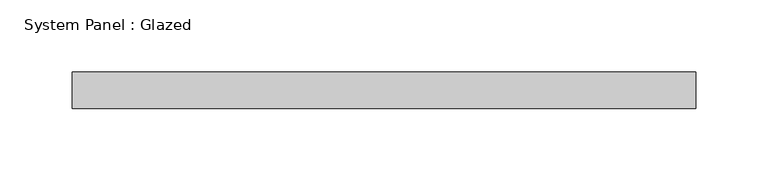
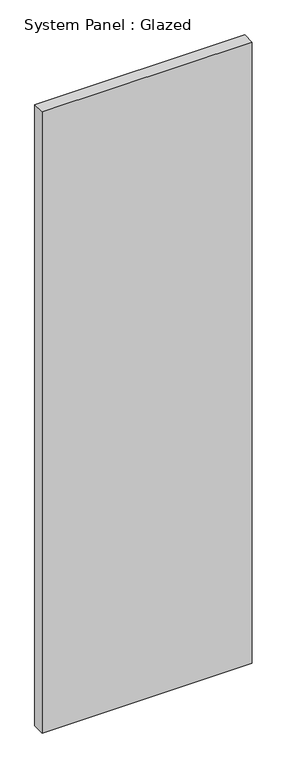
"""IFC4 building model written with IfcOpenShell, lengths in millimetres: plate geometry, System Panel : Glazed."""

from ifc_helpers import new_model, si_unit, origin, origin_with_axes, place, context, project, spatial, polyline, outline, extrude, source, transform, mapped, element, save


def system_panel_glazed_e1e129e0(model_context):
    return source(origin(), model_context, "Body", "SweptSolid", [
        extrude(outline(polyline([(215.9, 19.05), (-215.9, 19.05), (-215.9, 44.45), (215.9, 44.45), (215.9, 19.05)])), origin_with_axes(), (0.0, 0.0, 1.0), 1348.7821201),
    ])


if __name__ == "__main__":
    model = new_model("IFC4")
    model_context = context("Model", 3, world=origin())
    ifc_project = project(units=[si_unit("LENGTHUNIT", "METRE", prefix="MILLI")], contexts=[model_context])
    site = spatial("IfcSite", under=ifc_project)
    building = spatial("IfcBuilding", under=site)
    placement = place(None, origin())
    system_panel_glazed_shape = system_panel_glazed_e1e129e0(model_context)
    element("IfcPlate", 1, ObjectType="System Panel : Glazed", at=placement, inside=building, context=model_context, shape_type="MappedRepresentation", body=[
        mapped(system_panel_glazed_shape, transform((0.0, 0.0, 0.0), x_axis=(1.0, 0.0, 0.0), y_axis=(0.0, 1.0, 0.0), z_axis=(0.0, 0.0, 1.0))),
    ])
    save(model, "model.ifc")

# Revit data of these elements
# Type "System Panel : Glazed"
#   Construction Type Id = "GSP4R"
#   Analytic Construction = "1/8 in Pilkington single glazing"
#   Visual Light Transmittance = 0.9
#   Solar Heat Gain Coefficient = 0.86
#   Heat Transfer Coefficient (U) = 1.18115 BTU/(h·ft²·°F)
#   Define Thermal Properties by = 1
# Element 1 (IfcPlate, "System Panel : Glazed")
#   Materials on its faces: "Glass"
# Materials
#   "Glass": class "Glass", colour RGB 0 128 192, transparency 0.75, Description = "Soda Lime Glass", Cost = 0
